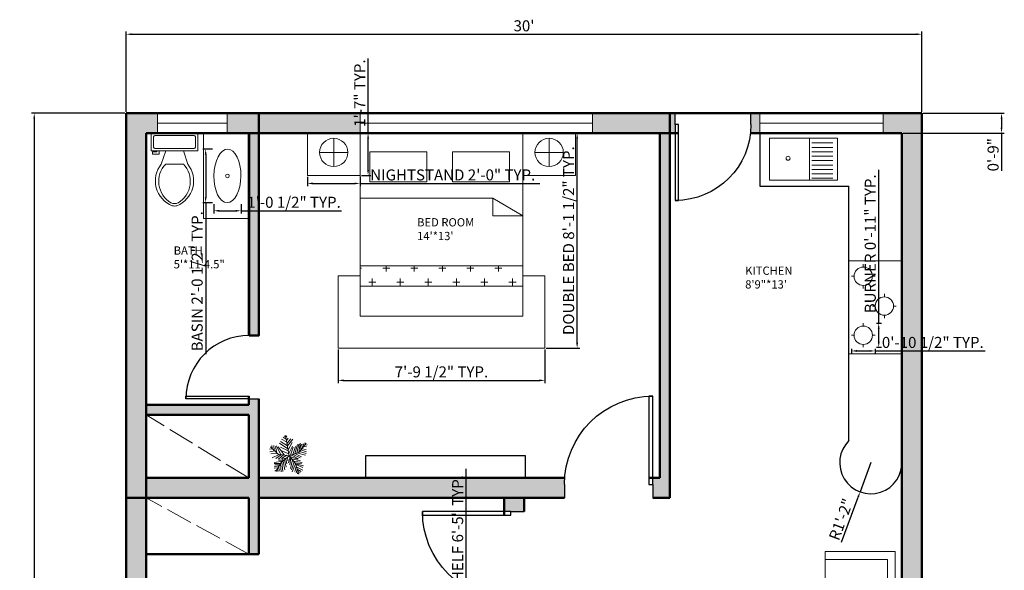
# Model space of a CAD drawing. Units: inches. Extents: x 1864 to 2313, y 963 to 1675.
# Tile 2 of 2: x 1868 to 2313, y 1425 to 1675. Entities that reach past the tile are written whole.
import ezdxf

# ---------------------------------------------------------------- set-up
doc = ezdxf.new("R2010")
doc.units = ezdxf.units.IN
doc.linetypes.add('ACAD_ISO02W100', pattern=[15, 12, -3])
for name, color, linetype, lineweight in [('A-ANNO-DIMS', 210, 'Continuous', 18), ('A-AREA-IDEN', 210, 'Continuous', 18), ('A-EQPM', 230, 'Continuous', 18), ('A-FLOR-CASE', 230, 'Continuous', 25), ('A-FLOR-CASE-OVHD', 142, 'ACAD_ISO02W100', 18), ('A-FLOR-FIXT', 40, 'Continuous', 18), ('A-FURN-PATT', 40, 'Continuous', 13), ('A-WALL-PATT', 142, 'Continuous', 13), ('door', 50, 'Continuous', 25), ('fur', 40, 'Continuous', 18), ('tree', 90, 'Continuous', 18), ('wall', 7, 'Continuous', 50), ('wind', 201, 'Continuous', 20)]:
    doc.layers.add(name, color=color, linetype=linetype, lineweight=lineweight)
doc.styles.get("Standard").update_dxf_attribs({"font": 'arial.ttf'})
doc.dimstyles.new('ISO-25', dxfattribs={"dimtxt": 5, "dimasz": 2.5, "dimexe": 1.25, "dimexo": 0.625, "dimtad": 1, "dimdec": 0, "dimlunit": 4, "dimtxsty": 'Standard', "dimcen": 2.5, "dimadec": 0, "dimazin": 0, "dimtfac": 1, "dimtdec": 0, "dimtmove": 0, "dimatfit": 3, "dimfxl": 1, "dimarcsym": 0})

# ---------------------------------------------------------------- blocks, each defined once
blk = doc.blocks.new('*U2')
for p, q in [((0, 0), (0, -6)), ((40, 0), (40, -6))]:
    blk.add_line(p, q)
blk.add_lwpolyline([(0, 0), (0, 40), (1.75, 40), (1.75, 0)], close=True)
blk.add_arc((0, 0), 40, 0, 90)
blk = doc.blocks.new('*U4')
for p, q in [((9.5, -6), (9.5, -2)), ((-10, -8.5), (-8, -8.5)), ((-10, -9.5), (-10, -8.5)), ((-8, -8.5), (-8, -8)), ((-7, -8), (-7, -9.5)), ((-4, -8), (-6, -14)), ((4, -8), (6, -14)), ((-7, -9.5), (-10, -9.5)), ((4, -14), (-4, -14))]:
    blk.add_line(p, q)
blk.add_lwpolyline([(10.5, -8), (10.5, 0), (-10.5, 0), (-10.5, -8)], close=True)
for points in [[(-9.5, -2), (-9.5, -6)], [(8.5, -1), (-8.5, -1)], [(-8.5, -7), (8.5, -7)]]:
    blk.add_lwpolyline(points)
for centre, radius, start, end in [((-8.62, -1.88), 0.884, 81.8699, 188.1301), ((8.62, -1.88), 0.884, 351.8699, 98.1301), ((-8.62, -6.12), 0.884, 171.8699, 278.1301), ((8.62, -6.12), 0.884, 261.8699, 8.1301), ((3.52, -21.58), 12.17, 141.4691, 247.9714), ((4.2, -21.82), 11.33, 136.3677, 238.9468), ((-3.52, -21.58), 12.17, 292.0284, 38.5307), ((-4.2, -21.82), 11.33, 301.053, 43.6321), ((0, -27.88), 4, 245.7318, 294.2682), ((0, -29), 4, 254.8605, 285.1395)]:
    blk.add_arc(centre, radius, start, end)
blk = doc.blocks.new('*U8')
for p, q in [((-10.186, 53.64), (-13.084, 55.962)), ((0, 0), (-10.5, 57)), ((-9.099, 51.782), (-6.563, 55.962)), ((-48.585, 21.131), (-49.309, 29.026)), ((-43.513, 28.561), (-42.427, 15.558)), ((-35.544, 28.097), (-24.314, 3.947)), ((-3.665, 19.273), (-27.574, 35.527)), ((-5.114, 28.097), (-24.676, 40.636)), ((-7.288, 39.707), (-21.778, 46.673)), ((-8.737, 47.138), (-17.069, 52.711)), ((-7.65, 43.423), (-2.578, 49.46)), ((-5.839, 35.992), (4.667, 48.067)), ((-5.114, 27.632), (10.463, 46.673)), ((-2.941, 16.486), (8.652, 37.85)), ((16.259, 5.805), (23.142, 31.348)), ((22.055, 7.198), (27.489, 32.277)), ((27, 9), (48, 36)), ((27.127, 9.056), (31.112, 35.992)), ((31.836, 30.883), (32.561, 16.486)), ((35.096, 32.741), (37.27, 22.524)), ((38.719, 34.134), (41.979, 28.561)), ((43.791, 29.954), (51.036, 30.883)), ((44.153, 36.456), (45.239, 32.741)), ((-47.498, 19.737), (-55.83, 18.344)), ((-40.615, 13.7), (-55.105, 10.913)), ((-31.5, 4.5), (-52.5, 25.5)), ((-33.37, 6.269), (-52.207, 5.34)), ((-28.299, 3.483), (-47.86, -5.805)), ((-38.442, 26.239), (-34.819, 7.663)), ((-21.416, 3.018), (-38.079, -8.128)), ((0, 0), (-31.5, 4.5)), ((-14.533, 2.09), (-30.834, 25.31)), ((-15.982, 2.09), (-30.11, -9.521)), ((-24.314, 23.917), (-2.941, 13.7)), ((0, 0), (-22.5, -19.5)), ((-6.563, 1.161), (-21.416, -8.128)), ((-20.691, 13.7), (-1.129, 4.876)), ((-1.129, 6.734), (9.014, 26.704)), ((0, 0), (27, 9)), ((0, 0), (18, -22.5)), ((3.942, 1.625), (11.187, 24.381)), ((6.478, 1.625), (26.04, -8.592)), ((10.101, 3.483), (17.708, 26.239)), ((11.187, 3.483), (30.749, -5.805)), ((18.07, 5.805), (35.096, -3.483)), ((24.229, 7.663), (46.688, 1.625)), ((29.662, 12.307), (48.137, 6.269)), ((33.285, 16.486), (48.862, 10.913)), ((36.183, 19.737), (48.137, 17.88)), ((40.53, 25.775), (48.862, 24.846)), ((-17.431, -15.094), (-42.789, -18.809)), ((-24.314, -21.596), (-42.427, -22.06)), ((-26.849, -26.24), (-40.253, -25.775)), ((-22.5, -19.5), (-37.5, -45)), ((-15.257, -12.772), (-30.11, -12.772)), ((-25.038, -23.918), (-22.865, -45.281)), ((-20.691, -18.345), (-17.793, -44.352)), ((-6.563, -5.805), (-19.967, -9.985)), ((-17.069, -15.094), (-12.721, -40.172)), ((-13.446, -11.378), (-8.737, -32.741)), ((-9.461, -8.592), (-6.201, -23.453)), ((-4.752, -3.483), (-3.665, -14.629)), ((2.493, -3.019), (-1.491, -20.202)), ((1.769, -2.555), (24.229, -9.521)), ((5.029, -6.27), (2.131, -25.775)), ((9.014, -11.378), (3.58, -35.992)), ((14.085, -16.951), (6.478, -40.172)), ((7.565, -9.056), (32.198, -14.629)), ((18.07, -22.524), (8.289, -45.745)), ((12.274, -15.094), (36.907, -18.809)), ((16.259, -19.738), (36.183, -22.989)), ((18, -22.5), (27, -52.5)), ((18.433, -22.524), (40.53, -29.026)), ((19.157, -25.311), (38.719, -33.206)), ((-28.299, -29.026), (-42.789, -31.348)), ((-30.834, -34.135), (-42.427, -35.528)), ((-34.457, -39.708), (-40.978, -42.494)), ((-32.646, -36.921), (-31.921, -44.352)), ((-29.023, -30.884), (-27.936, -43.887)), ((20.244, -30.419), (15.897, -44.816)), ((22.78, -37.85), (19.519, -48.532)), ((21.331, -32.741), (39.081, -40.636)), ((22.78, -38.314), (34.372, -44.816)), ((24.591, -45.745), (23.142, -50.854)), ((24.591, -43.423), (30.749, -47.603)), ((26.764, -49.925), (28.213, -50.854))]:
    blk.add_line(p, q)
blk = doc.blocks.new('*D9')
at = {"layer": 'A-ANNO-DIMS', "color": 0, "lineweight": -2, "transparency": 16777216}
for p, q in [((1915.95, 1632.78), (1915.95, 1669.17)), ((1918.45, 1667.92), (2273.45, 1667.92)), ((2275.95, 1632.78), (2275.95, 1669.17))]:
    blk.add_line(p, q, dxfattribs=at)
at = {"layer": 'A-ANNO-DIMS', "color": 0, "lineweight": 100, "transparency": 16777216}
for points in [[(1918.45, 1668.34), (1918.45, 1667.51), (1915.95, 1667.92)], [(2273.45, 1668.34), (2273.45, 1667.51), (2275.95, 1667.92)]]:
    blk.add_solid(points, dxfattribs=at)
at = {"layer": 'Defpoints', "color": 0, "lineweight": 100, "transparency": 16777216}
for p in [(2275.95, 1667.92), (1915.95, 1632.16), (2275.95, 1632.16)]:
    blk.add_point(p, dxfattribs=at)
at = {"layer": 'A-ANNO-DIMS', "color": 0, "transparency": 16777216, "insert": (2095.95, 1671.1), "char_height": 5, "attachment_point": 5}
blk.add_mtext("30'", dxfattribs=at)
blk = doc.blocks.new('*D10')
at = {"layer": 'A-ANNO-DIMS', "color": 0, "lineweight": -2, "transparency": 16777216}
for p, q in [((1915.33, 1632.16), (1873.06, 1632.16)), ((1874.31, 1629.66), (1874.31, 965.66)), ((1915.33, 963.16), (1873.06, 963.16))]:
    blk.add_line(p, q, dxfattribs=at)
at = {"layer": 'A-ANNO-DIMS', "color": 0, "lineweight": 100, "transparency": 16777216}
for points in [[(1873.89, 1629.66), (1874.73, 1629.66), (1874.31, 1632.16)], [(1873.89, 965.66), (1874.73, 965.66), (1874.31, 963.16)]]:
    blk.add_solid(points, dxfattribs=at)
at = {"layer": 'Defpoints', "color": 0, "lineweight": 100, "transparency": 16777216}
for p in [(1915.95, 1632.16), (1874.31, 963.16), (1915.95, 963.16)]:
    blk.add_point(p, dxfattribs=at)
at = {"layer": 'A-ANNO-DIMS', "color": 0, "transparency": 16777216, "insert": (1871.13, 1297.66), "char_height": 5, "attachment_point": 5, "rotation": 90}
blk.add_mtext('55\'-9"', dxfattribs=at)
blk = doc.blocks.new('BED-DOUBLE')
for p, q in [((10, 67.81), (70, 67.81)), ((70, 67.81), (70, 59.9)), ((83.6, 59.9), (70, 67.81)), ((70, 59.9), (83.6, 59.9)), ((5, 32.66), (0, 32.66)), ((0, 32.66), (0, 0)), ((10, 32.66), (5, 32.66)), ((83.6, 32.66), (93.6, 32.66)), ((93.6, 32.66), (93.6, 0)), ((0, 0), (93.6, 0))]:
    blk.add_line(p, q)
for points in [[(10, 97.3), (83.6, 97.3), (83.6, 14.55), (10, 14.55)], [(14.44, 88.9), (40.24, 88.9), (40.24, 75.28), (14.44, 75.28)], [(51.82, 88.9), (77.62, 88.9), (77.62, 75.28), (51.82, 75.28)]]:
    blk.add_lwpolyline(points, close=True)
blk = doc.blocks.new('TABLE-BEDSIDE')
for p, q in [((11.93, 4.03), (11.93, 16.85)), ((5.53, 10.44), (18.34, 10.44))]:
    blk.add_line(p, q)
blk.add_lwpolyline([(0, 19.17), (23.88, 19.17), (23.88, 0), (0, 0)], close=True)
blk.add_circle((11.93, 10.44), 6.41)
blk = doc.blocks.new('LOUNGE-CHAIR')
for p, q in [((3.79, 31.54), (0, 31.54)), ((0, 31.54), (0, 0)), ((3.79, 3.47), (3.79, 31.54)), ((30.24, 31.54), (33.95, 31.54)), ((33.95, 31.54), (33.95, 0)), ((0, 0), (33.95, 0))]:
    blk.add_line(p, q)
blk.add_lwpolyline([(3.79, 31.54), (30.24, 31.54), (30.24, 3.47), (3.79, 3.47)])
blk = doc.blocks.new('BASIN-OVAL')
blk.add_circle((12.11, 6.1), 0.811)
blk.add_ellipse((12.11, 6.1), major_axis=(12.1, -0.16), ratio=0.504372)
blk = doc.blocks.new('COOKTOP-BURNER')
for p, q in [((5.36, 10.94), (5.36, 9.63)), ((0, 5.47), (1.19, 5.47)), ((9.52, 5.47), (10.71, 5.47)), ((5.36, 1.31), (5.36, 0))]:
    blk.add_line(p, q)
blk.add_circle((5.36, 5.47), 4.16)
blk = doc.blocks.new('*D18')
at = {"layer": 'A-ANNO-DIMS', "color": 0, "lineweight": -2, "transparency": 16777216}
for p, q in [((1997.91, 1603.36), (1997.91, 1599.15)), ((2000.41, 1600.4), (2019.29, 1600.4)), ((2021.79, 1603.36), (2021.79, 1599.15)), ((2021.79, 1600.4), (2103.12, 1600.4))]:
    blk.add_line(p, q, dxfattribs=at)
at = {"layer": 'A-ANNO-DIMS', "color": 0, "lineweight": 100, "transparency": 16777216}
for points in [[(2000.41, 1600.82), (2000.41, 1599.99), (1997.91, 1600.4)], [(2019.29, 1600.82), (2019.29, 1599.99), (2021.79, 1600.4)]]:
    blk.add_solid(points, dxfattribs=at)
at = {"layer": 'Defpoints', "color": 0, "lineweight": 100, "transparency": 16777216}
for p in [(1997.91, 1603.99), (2021.79, 1603.99), (2021.79, 1600.4)]:
    blk.add_point(p, dxfattribs=at)
at = {"layer": 'A-ANNO-DIMS', "color": 0, "transparency": 16777216, "insert": (2063.71, 1603.61), "char_height": 5, "attachment_point": 5}
blk.add_mtext('NIGHTSTAND 2\'-0" TYP.', dxfattribs=at)
blk = doc.blocks.new('*D19')
at = {"layer": 'A-ANNO-DIMS', "color": 0, "lineweight": -2, "transparency": 16777216}
for p, q in [((2025.38, 1623.16), (2025.38, 1656.91)), ((2022.42, 1623.16), (2026.63, 1623.16)), ((2025.38, 1606.49), (2025.38, 1620.66)), ((2022.42, 1603.99), (2026.63, 1603.99))]:
    blk.add_line(p, q, dxfattribs=at)
at = {"layer": 'A-ANNO-DIMS', "color": 0, "lineweight": 100, "transparency": 16777216}
for points in [[(2024.96, 1620.66), (2025.79, 1620.66), (2025.38, 1623.16)], [(2024.96, 1606.49), (2025.79, 1606.49), (2025.38, 1603.99)]]:
    blk.add_solid(points, dxfattribs=at)
at = {"layer": 'Defpoints', "color": 0, "lineweight": 100, "transparency": 16777216}
for p in [(2021.79, 1623.16), (2025.38, 1623.16), (2021.79, 1603.99)]:
    blk.add_point(p, dxfattribs=at)
at = {"layer": 'A-ANNO-DIMS', "color": 0, "transparency": 16777216, "insert": (2022.24, 1641.28), "char_height": 5, "attachment_point": 5, "rotation": 90}
blk.add_mtext('1\'-7" TYP.', dxfattribs=at)
blk = doc.blocks.new('*D20')
at = {"layer": 'A-ANNO-DIMS', "color": 0, "lineweight": -2, "transparency": 16777216}
for p, q in [((2256.46, 1537.18), (2256.46, 1606.51)), ((2255.45, 1537.18), (2257.71, 1537.18)), ((2256.46, 1528.74), (2256.46, 1534.68)), ((2255.45, 1526.24), (2257.71, 1526.24))]:
    blk.add_line(p, q, dxfattribs=at)
at = {"layer": 'A-ANNO-DIMS', "color": 0, "lineweight": 100, "transparency": 16777216}
for points in [[(2256.05, 1534.68), (2256.88, 1534.68), (2256.46, 1537.18)], [(2256.05, 1528.74), (2256.88, 1528.74), (2256.46, 1526.24)]]:
    blk.add_solid(points, dxfattribs=at)
at = {"layer": 'Defpoints', "color": 0, "lineweight": 100, "transparency": 16777216}
for p in [(2254.82, 1537.18), (2256.46, 1537.18), (2254.82, 1526.24)]:
    blk.add_point(p, dxfattribs=at)
at = {"layer": 'A-ANNO-DIMS', "color": 0, "transparency": 16777216, "insert": (2253.29, 1573.09), "char_height": 5, "attachment_point": 5, "rotation": 90}
blk.add_mtext('BURNER 0\'-11" TYP.', dxfattribs=at)
blk = doc.blocks.new('*D21')
at = {"layer": 'A-ANNO-DIMS', "color": 0, "lineweight": -2, "transparency": 16777216}
for p, q in [((2244.11, 1525.62), (2244.11, 1523.35)), ((2246.61, 1524.6), (2252.32, 1524.6)), ((2254.82, 1525.62), (2254.82, 1523.35)), ((2254.82, 1524.6), (2304.59, 1524.6))]:
    blk.add_line(p, q, dxfattribs=at)
at = {"layer": 'A-ANNO-DIMS', "color": 0, "lineweight": 100, "transparency": 16777216}
for points in [[(2246.61, 1525.02), (2246.61, 1524.18), (2244.11, 1524.6)], [(2252.32, 1525.02), (2252.32, 1524.18), (2254.82, 1524.6)]]:
    blk.add_solid(points, dxfattribs=at)
at = {"layer": 'Defpoints', "color": 0, "lineweight": 100, "transparency": 16777216}
for p in [(2244.11, 1526.24), (2254.82, 1526.24), (2254.82, 1524.6)]:
    blk.add_point(p, dxfattribs=at)
at = {"layer": 'A-ANNO-DIMS', "color": 0, "transparency": 16777216, "insert": (2280.95, 1527.81), "char_height": 5, "attachment_point": 5}
blk.add_mtext('0\'-10 1/2" TYP.', dxfattribs=at)
blk = doc.blocks.new('*D22')
at = {"layer": 'A-ANNO-DIMS', "color": 0, "lineweight": -2, "transparency": 16777216}
for p, q in [((2106.01, 1623.16), (2121.23, 1623.16)), ((2119.98, 1528.36), (2119.98, 1620.66)), ((2106.01, 1525.86), (2121.23, 1525.86))]:
    blk.add_line(p, q, dxfattribs=at)
at = {"layer": 'A-ANNO-DIMS', "color": 0, "lineweight": 100, "transparency": 16777216}
for points in [[(2119.56, 1620.66), (2120.4, 1620.66), (2119.98, 1623.16)], [(2119.56, 1528.36), (2120.4, 1528.36), (2119.98, 1525.86)]]:
    blk.add_solid(points, dxfattribs=at)
at = {"layer": 'Defpoints', "color": 0, "lineweight": 100, "transparency": 16777216}
for p in [(2105.39, 1623.16), (2119.98, 1623.16), (2105.39, 1525.86)]:
    blk.add_point(p, dxfattribs=at)
at = {"layer": 'A-ANNO-DIMS', "color": 0, "transparency": 16777216, "insert": (2116.77, 1574.51), "char_height": 5, "attachment_point": 5, "rotation": 90}
blk.add_mtext('DOUBLE BED 8\'-1 1/2" TYP.', dxfattribs=at)
blk = doc.blocks.new('*D23')
at = {"layer": 'A-ANNO-DIMS', "color": 0, "lineweight": -2, "transparency": 16777216}
for p, q in [((2011.79, 1525.24), (2011.79, 1510.02)), ((2105.39, 1525.24), (2105.39, 1510.02)), ((2014.29, 1511.27), (2102.89, 1511.27))]:
    blk.add_line(p, q, dxfattribs=at)
at = {"layer": 'A-ANNO-DIMS', "color": 0, "lineweight": 100, "transparency": 16777216}
for points in [[(2014.29, 1511.69), (2014.29, 1510.85), (2011.79, 1511.27)], [(2102.89, 1511.69), (2102.89, 1510.85), (2105.39, 1511.27)]]:
    blk.add_solid(points, dxfattribs=at)
at = {"layer": 'Defpoints', "color": 0, "lineweight": 100, "transparency": 16777216}
for p in [(2011.79, 1525.86), (2105.39, 1525.86), (2105.39, 1511.27)]:
    blk.add_point(p, dxfattribs=at)
at = {"layer": 'A-ANNO-DIMS', "color": 0, "transparency": 16777216, "insert": (2058.59, 1514.48), "char_height": 5, "attachment_point": 5}
blk.add_mtext('7\'-9 1/2" TYP.', dxfattribs=at)
blk = doc.blocks.new('*D28')
at = {"layer": 'A-ANNO-DIMS', "color": 0, "lineweight": -2, "transparency": 16777216}
for p, q in [((1954.91, 1615.97), (1950.64, 1615.97)), ((1951.89, 1613.47), (1951.89, 1594.17)), ((1954.91, 1591.67), (1950.64, 1591.67)), ((1951.89, 1591.67), (1951.89, 1523.11))]:
    blk.add_line(p, q, dxfattribs=at)
at = {"layer": 'A-ANNO-DIMS', "color": 0, "lineweight": 100, "transparency": 16777216}
for points in [[(1951.48, 1613.47), (1952.31, 1613.47), (1951.89, 1615.97)], [(1951.48, 1594.17), (1952.31, 1594.17), (1951.89, 1591.67)]]:
    blk.add_solid(points, dxfattribs=at)
at = {"layer": 'Defpoints', "color": 0, "lineweight": 100, "transparency": 16777216}
for p in [(1955.54, 1615.97), (1951.89, 1591.67), (1955.54, 1591.67)]:
    blk.add_point(p, dxfattribs=at)
at = {"layer": 'A-ANNO-DIMS', "color": 0, "transparency": 16777216, "insert": (1948.68, 1556.14), "char_height": 5, "attachment_point": 5, "rotation": 90}
blk.add_mtext('BASIN 2\'-0 1/2" TYP.', dxfattribs=at)
blk = doc.blocks.new('*D29')
at = {"layer": 'A-ANNO-DIMS', "color": 0, "lineweight": -2, "transparency": 16777216}
for p, q in [((1955.54, 1591.05), (1955.54, 1586.78)), ((1967.93, 1591.05), (1967.93, 1586.78)), ((1958.04, 1588.03), (1965.43, 1588.03)), ((1967.93, 1588.03), (2013.33, 1588.03))]:
    blk.add_line(p, q, dxfattribs=at)
at = {"layer": 'A-ANNO-DIMS', "color": 0, "lineweight": 100, "transparency": 16777216}
for points in [[(1958.04, 1588.44), (1958.04, 1587.61), (1955.54, 1588.03)], [(1965.43, 1588.44), (1965.43, 1587.61), (1967.93, 1588.03)]]:
    blk.add_solid(points, dxfattribs=at)
at = {"layer": 'Defpoints', "color": 0, "lineweight": 100, "transparency": 16777216}
for p in [(1955.54, 1591.67), (1967.93, 1591.67), (1967.93, 1588.03)]:
    blk.add_point(p, dxfattribs=at)
at = {"layer": 'A-ANNO-DIMS', "color": 0, "transparency": 16777216, "insert": (1991.88, 1591.24), "char_height": 5, "attachment_point": 5}
blk.add_mtext('1\'-0 1/2" TYP.', dxfattribs=at)
blk = doc.blocks.new('*D30')
at = {"layer": 'A-ANNO-DIMS', "color": 0, "lineweight": -2, "transparency": 16777216}
for p, q in [((2069.78, 1391.45), (2069.78, 1471.3)), ((2080.73, 1391.45), (2068.53, 1391.45)), ((2069.78, 1316.78), (2069.78, 1388.95)), ((2080.73, 1314.28), (2068.53, 1314.28))]:
    blk.add_line(p, q, dxfattribs=at)
at = {"layer": 'A-ANNO-DIMS', "color": 0, "lineweight": 100, "transparency": 16777216}
for points in [[(2069.36, 1388.95), (2070.19, 1388.95), (2069.78, 1391.45)], [(2069.36, 1316.78), (2070.19, 1316.78), (2069.78, 1314.28)]]:
    blk.add_solid(points, dxfattribs=at)
at = {"layer": 'Defpoints', "color": 0, "lineweight": 100, "transparency": 16777216}
for p in [(2069.78, 1391.45), (2081.35, 1391.45), (2081.35, 1314.28)]:
    blk.add_point(p, dxfattribs=at)
at = {"layer": 'A-ANNO-DIMS', "color": 0, "transparency": 16777216, "insert": (2066.57, 1432.63), "char_height": 5, "attachment_point": 5, "rotation": 90}
blk.add_mtext('WALL SHELF 6\'-5" TYP.', dxfattribs=at)
blk = doc.blocks.new('*D32')
at = {"layer": 'A-ANNO-DIMS', "color": 0, "lineweight": -2, "transparency": 16777216}
for p, q in [((2276.58, 1632.16), (2313.3, 1632.16)), ((2312.05, 1629.66), (2312.05, 1625.66)), ((2267.58, 1623.16), (2313.3, 1623.16)), ((2312.05, 1623.16), (2312.05, 1606.11))]:
    blk.add_line(p, q, dxfattribs=at)
at = {"layer": 'A-ANNO-DIMS', "color": 0, "lineweight": 100, "transparency": 16777216}
for points in [[(2311.64, 1629.66), (2312.47, 1629.66), (2312.05, 1632.16)], [(2311.64, 1625.66), (2312.47, 1625.66), (2312.05, 1623.16)]]:
    blk.add_solid(points, dxfattribs=at)
at = {"layer": 'Defpoints', "color": 0, "lineweight": 100, "transparency": 16777216}
for p in [(2275.95, 1632.16), (2266.95, 1623.16), (2312.05, 1623.16)]:
    blk.add_point(p, dxfattribs=at)
at = {"layer": 'A-ANNO-DIMS', "color": 0, "transparency": 16777216, "insert": (2308.88, 1613.39), "char_height": 5, "attachment_point": 5, "rotation": 90}
blk.add_mtext('0\'-9"', dxfattribs=at)
blk = doc.blocks.new('*D33')
at = {"layer": 'A-ANNO-DIMS', "color": 0, "lineweight": -2, "transparency": 16777216}
for p, q in [((2252.91, 1474.05), (2248.04, 1460.83)), ((2239.64, 1438), (2247.18, 1458.48))]:
    blk.add_line(p, q, dxfattribs=at)
at = {"layer": 'A-ANNO-DIMS', "color": 0, "lineweight": 100, "transparency": 16777216}
blk.add_solid([(2246.79, 1458.63), (2247.57, 1458.34), (2248.04, 1460.83)], dxfattribs=at)
at = {"layer": 'Defpoints', "color": 0, "lineweight": 100, "transparency": 16777216}
for p in [(2252.91, 1474.05), (2248.04, 1460.83)]:
    blk.add_point(p, dxfattribs=at)
at = {"layer": 'A-ANNO-DIMS', "color": 0, "transparency": 16777216, "insert": (2240.03, 1448.15), "char_height": 5, "attachment_point": 5, "rotation": 69.7872}
blk.add_mtext('R1\'-2"', dxfattribs=at)

msp = doc.modelspace()

# ---------------------------------------------------------------- hatches: boundary and pattern name
at = {"layer": 'A-FURN-PATT'}
h = msp.add_hatch(dxfattribs=at)
h.set_pattern_fill('CROSS', color=256)
h.paths.add_polyline_path([(2095.39, 1563.09), (2021.79, 1563.09), (2021.79, 1553.95), (2095.39, 1553.95)])
at = {"layer": 'A-WALL-PATT'}
h = msp.add_hatch(color=256, dxfattribs=at)
h.dxf.hatch_style = 1
h.paths.add_polyline_path([(1975.95, 1632.16), (1961.64, 1632.16), (1961.64, 1623.16), (1971.45, 1623.16), (1975.95, 1623.16)])
h.paths.add_polyline_path([(2021.79, 1632.16), (1989.45, 1632.16), (1975.95, 1632.16), (1975.95, 1623.16), (1984.95, 1623.16), (1989.45, 1623.16), (2021.79, 1623.16)])
h.paths.add_polyline_path([(2161.95, 1632.16), (2126.93, 1632.16), (2126.93, 1623.16), (2157.45, 1623.16), (2161.95, 1623.16)])
h.paths.add_polyline_path([(2275.95, 1632.16), (2258.45, 1632.16), (2258.45, 1623.16), (2266.95, 1623.16), (2266.95, 1475.18, -0.040334), (2266.95, 1472.91), (2266.95, 1467.16), (2266.95, 1458.16), (2266.95, 1278.16), (2266.95, 1269.16), (2275.95, 1269.16), (2275.95, 1458.16)])
h.paths.add_polyline_path([(2161.95, 1623.16), (2157.45, 1623.16), (2157.45, 1467.16), (2154.26, 1467.16), (2154.26, 1464.16), (2154.26, 1458.16), (2161.95, 1458.16)])
h.paths.add_polyline_path([(2202.62, 1632.16), (2198.67, 1632.16), (2198.67, 1627.01, -0.028105), (2198.46, 1623.16), (2202.62, 1623.16)])
h.paths.add_polyline_path([(2164.34, 1627.01), (2164.34, 1632.16), (2161.95, 1632.16), (2161.95, 1623.16), (2164.34, 1623.16)])
h.paths.add_polyline_path([(1930.16, 1632.16), (1929.45, 1632.16), (1915.95, 1632.16), (1915.95, 1458.16), (1924.95, 1458.16), (1924.95, 1623.16), (1930.16, 1623.16)])
h.paths.add_polyline_path([(1924.95, 1441.66), (1924.95, 1458.16), (1915.95, 1458.16), (1915.95, 1285.66), (1924.95, 1285.66)])
h.paths.add_polyline_path([(2044.94, 1221.16), (2037.45, 1221.16), (1924.95, 1221.16), (1924.95, 1216.66), (2044.94, 1216.66)])
h.paths.add_polyline_path([(2037.45, 1234.15), (2032.95, 1234.15), (2032.95, 1221.16), (2037.45, 1221.16)])
h.paths.add_polyline_path([(2086.95, 1221.16), (2076.95, 1221.16), (2076.95, 1216.66), (2086.95, 1216.66)])
h.paths.add_polyline_path([(2107.14, 1185.16), (2095.95, 1185.16), (2095.95, 1189.94), (2092.08, 1189.94, -0.049915), (2086.95, 1190.46), (2086.95, 1176.16), (2107.14, 1176.16), (2107.14, 1178.61)])
h.paths.add_polyline_path([(2095.95, 1176.16), (2086.95, 1176.16), (2086.95, 1056.16), (2086.95, 1039.66), (2095.95, 1039.66), (2095.95, 1056.16)])
h.paths.add_polyline_path([(2086.95, 1048.66), (2057.44, 1048.66), (2057.44, 1039.66), (2086.95, 1039.66)])
h.paths.add_polyline_path([(1959.08, 1048.66), (1915.95, 1048.66), (1915.95, 1039.66), (1920.45, 1039.66), (1959.08, 1039.66)])
h.paths.add_polyline_path([(1924.95, 1216.66), (1924.95, 1221.16), (1915.95, 1221.16), (1915.95, 1048.66), (1924.95, 1048.66)])
h.paths.add_polyline_path([(1924.95, 1281.16), (1924.95, 1285.66), (1915.95, 1285.66), (1915.95, 1221.16), (1924.95, 1221.16)])
h.paths.add_polyline_path([(2037.45, 1285.66), (2028.44, 1285.66), (2028.44, 1281.58), (2028.44, 1281.16), (2032.95, 1281.16), (2032.95, 1272.41), (2037.45, 1272.41)])
h.paths.add_polyline_path([(2045.26, 1285.66), (2037.45, 1285.66), (2037.45, 1281.16), (2045.26, 1281.16)])
h.paths.add_polyline_path([(2086.95, 1285.66), (2080.03, 1285.66), (2080.03, 1281.16), (2086.95, 1281.16)])
h.paths.add_polyline_path([(2095.95, 1269.16), (2086.95, 1269.16), (2086.95, 1215.79), (2092.08, 1215.79), (2095.95, 1215.79)])
h = msp.add_hatch(color=256, dxfattribs=at)
h.dxf.hatch_style = 1
h.paths.add_polyline_path([(1975.95, 1623.16), (1971.64, 1623.16), (1971.64, 1531.6), (1975.95, 1531.6)])
h = msp.add_hatch(color=256, dxfattribs=at)
h.dxf.hatch_style = 1
h.paths.add_polyline_path([(1975.95, 1502.87), (1971.45, 1502.87), (1971.45, 1500.16), (1924.95, 1500.16), (1924.95, 1495.66), (1971.45, 1495.66), (1971.45, 1467.16), (1924.95, 1467.16), (1924.95, 1458.16), (1971.45, 1458.16), (1971.45, 1432.56), (1975.95, 1432.56), (1975.95, 1467.16)])
h.paths.add_polyline_path([(2114.37, 1467.16), (1975.95, 1467.16), (1975.95, 1458.16), (2114.26, 1458.16), (2114.26, 1464.16, -0.01877)])
h.paths.add_polyline_path([(2095.95, 1458.16), (2086.95, 1458.16), (2086.95, 1451.99), (2089.95, 1451.99), (2095.95, 1451.99)])

# ---------------------------------------------------------------- linework, layer by layer
at = {"layer": 'A-EQPM'}
msp.add_lwpolyline([(2266.95, 1565.31), (2242.95, 1565.31), (2242.95, 1523.35), (2266.95, 1523.35)], close=True, dxfattribs=at)
at = {"layer": 'A-FLOR-CASE'}
for p, q in [((2202.62, 1623.16), (2202.62, 1599.16)), ((2202.62, 1599.16), (2242.95, 1599.16)), ((2242.95, 1484.02), (2242.95, 1599.16))]:
    msp.add_line(p, q, dxfattribs=at)
msp.add_lwpolyline([(2024.23, 1467.16), (2096.59, 1467.16), (2096.59, 1477.17), (2024.23, 1477.17)], close=True, dxfattribs=at)
msp.add_arc((2252.91, 1474.05), 14.09, 134.9578, 4.6195, dxfattribs=at)
at = {"layer": 'A-FLOR-CASE-OVHD'}
for p, q in [((1971.45, 1467.16), (1924.95, 1495.66)), ((1971.45, 1432.56), (1924.95, 1458.16))]:
    msp.add_line(p, q, dxfattribs=at)
at = {"layer": 'A-FLOR-FIXT'}
for p, q in [((2225.19, 1601.88), (2225.19, 1620.84)), ((2226.15, 1618.72), (2235.74, 1618.72)), ((2226.15, 1616.72), (2235.74, 1616.72)), ((2226.15, 1614.72), (2235.74, 1614.72)), ((2226.15, 1612.72), (2235.74, 1612.72)), ((2226.15, 1610.72), (2235.74, 1610.72)), ((2226.15, 1608.72), (2235.74, 1608.72)), ((2226.15, 1606.72), (2235.74, 1606.72)), ((2226.15, 1604.72), (2235.74, 1604.72)), ((2226.15, 1602.72), (2235.74, 1602.72))]:
    msp.add_line(p, q, dxfattribs=at)
for points in [[(1971.45, 1623.16), (1971.45, 1584.47), (1950.84, 1584.47), (1950.84, 1623.16)], [(2207.04, 1620.84), (2237.78, 1620.84), (2237.78, 1601.88), (2207.04, 1601.88)]]:
    msp.add_lwpolyline(points, close=True, dxfattribs=at)
msp.add_circle((2215.43, 1611.82), 0.917, dxfattribs=at)
at = {"layer": 'fur'}
msp.add_lwpolyline([(2021.79, 1553.95), (2095.39, 1553.95), (2095.39, 1563.09), (2021.79, 1563.09)], close=True, dxfattribs=at)
at = {"layer": 'wall'}
for p, q in [((1915.95, 1495.66), (1915.95, 1632.16)), ((1915.95, 1285.66), (1915.95, 1632.16)), ((1915.95, 1632.16), (1929.45, 1632.16)), ((1929.45, 1632.16), (1989.45, 1632.16)), ((1975.95, 1632.16), (1975.95, 1531.6)), ((1989.45, 1632.16), (2161.95, 1632.16)), ((2161.95, 1632.16), (2161.95, 1458.16)), ((2161.95, 1632.16), (2275.95, 1632.16)), ((2275.95, 1632.16), (2275.95, 1458.16)), ((1924.95, 1623.16), (1984.95, 1623.16)), ((1924.95, 1500.16), (1924.95, 1623.16)), ((1924.95, 1281.16), (1924.95, 1623.16)), ((1971.45, 1623.16), (1971.45, 1531.6)), ((1975.95, 1623.16), (1975.95, 1531.6)), ((1984.95, 1623.16), (1989.45, 1623.16)), ((1989.45, 1623.16), (2157.45, 1623.16)), ((2157.45, 1623.16), (2157.45, 1467.16)), ((2157.45, 1623.16), (2161.95, 1623.16)), ((2161.95, 1623.16), (2165.84, 1623.16)), ((2198.46, 1623.16), (2266.95, 1623.16)), ((2266.95, 1623.16), (2266.95, 1467.16)), ((1971.45, 1504.13), (1971.45, 1500.16)), ((1975.95, 1502.87), (1975.95, 1467.16)), ((1975.95, 1502.87), (1975.95, 1495.66)), ((1971.45, 1500.16), (1924.95, 1500.16)), ((1915.95, 1495.66), (1915.95, 1458.16)), ((1971.45, 1495.66), (1924.95, 1495.66)), ((1924.95, 1495.66), (1924.95, 1467.16)), ((1971.45, 1467.16), (1971.45, 1495.66)), ((1975.95, 1467.16), (1975.95, 1495.66)), ((1971.45, 1467.16), (1971.45, 1472.45)), ((1975.95, 1467.16), (1975.95, 1472.45)), ((1971.45, 1467.16), (1924.95, 1467.16)), ((1975.95, 1467.16), (1975.95, 1432.56)), ((2114.37, 1467.16), (1975.95, 1467.16)), ((2157.45, 1467.16), (2152.51, 1467.16)), ((2266.95, 1467.16), (2266.95, 1458.16)), ((1971.45, 1458.16), (1915.95, 1458.16)), ((1971.45, 1458.16), (1971.45, 1432.56)), ((2114.26, 1458.16), (1975.95, 1458.16)), ((2086.95, 1450.24), (2086.95, 1458.16)), ((2095.95, 1451.99), (2095.95, 1458.16)), ((2161.95, 1458.16), (2154.26, 1458.16)), ((2266.95, 1458.16), (2266.95, 1278.16)), ((2275.95, 1458.16), (2275.95, 1269.16)), ((1924.95, 1285.66), (1924.95, 1441.66)), ((1971.45, 1432.56), (1924.95, 1432.56)), ((1927.7, 1432.56), (1924.95, 1432.56)), ((1975.95, 1432.56), (1971.45, 1432.56))]:
    msp.add_line(p, q, dxfattribs=at)
msp.add_lwpolyline([(1971.64, 1623.16), (1975.95, 1623.16), (1975.95, 1531.6), (1971.64, 1531.6)], close=True, dxfattribs=at)
at = {"layer": 'wind'}
for p, q in [((1930.16, 1627.66), (1961.64, 1627.66)), ((2021.79, 1627.66), (2126.93, 1627.66)), ((2202.62, 1627.66), (2258.45, 1627.66))]:
    msp.add_line(p, q, dxfattribs=at)
for points in [[(1930.16, 1623.16), (1961.64, 1623.16), (1961.64, 1632.16), (1930.16, 1632.16)], [(2021.79, 1623.16), (2126.93, 1623.16), (2126.93, 1632.16), (2021.79, 1632.16)], [(2258.45, 1632.16), (2202.62, 1632.16), (2202.62, 1623.16), (2258.45, 1623.16)]]:
    msp.add_lwpolyline(points, close=True, dxfattribs=at)

# ---------------------------------------------------------------- block references
at = {"layer": 'A-EQPM'}
for p in [(2244.11, 1552.92), (2253.67, 1539.46), (2244.11, 1526.24)]:
    msp.add_blockref('COOKTOP-BURNER', p, dxfattribs=at)
at = {"layer": 'A-FLOR-FIXT'}
msp.add_blockref('*U4', (1937.79, 1623.16), dxfattribs=at)
at = {"layer": 'A-FLOR-FIXT', "rotation": 269.9999999999978}
msp.add_blockref('BASIN-OVAL', (1955.63, 1615.93), dxfattribs=at)
at = {"layer": 'door'}
for p, xscale, yscale, zscale, rotation in [((2164.34, 1627.01), -0.858268468651503, 0.858268468651503, 0.858268468651503, 180), ((1971.64, 1502.87), 0.718277175322918, 0.718277175322918, 0.718277175322918, 90)]:
    msp.add_blockref('*U2', p, dxfattribs=dict(at, xscale=xscale, yscale=yscale, zscale=zscale, rotation=rotation))
at = {"layer": 'door', "xscale": -1}
msp.add_blockref('*U2', (2154.26, 1464.16), dxfattribs=at)
at = {"layer": 'door', "xscale": -1, "rotation": 90}
msp.add_blockref('*U2', (2089.95, 1451.99), dxfattribs=at)
at = {"layer": 'fur'}
for name, p in [('TABLE-BEDSIDE', (1997.91, 1603.99)), ('BED-DOUBLE', (2011.79, 1525.86)), ('TABLE-BEDSIDE', (2095.39, 1603.99))]:
    msp.add_blockref(name, p, dxfattribs=at)
at = {"layer": 'fur', "rotation": 89.99999999999964}
msp.add_blockref('LOUNGE-CHAIR', (2263.85, 1399.95), dxfattribs=at)
at = {"layer": 'tree', "xscale": 0.1597188363102572, "yscale": 0.1597188363102572, "zscale": 0.1597188363102572}
msp.add_blockref('*U8', (1989.68, 1477.18), dxfattribs=at)

# ---------------------------------------------------------------- texts
at = {"layer": 'A-AREA-IDEN', "char_height": 3.726, "attachment_point": 1}
for s, insert in [("BED ROOM\\P14'*13'", (2047.57, 1584.69)), ('BATH\\P5\'*11\'4.5"', (1937.41, 1571.9)), ('KITCHEN\\P8\'9"*13\'', (2196.04, 1562.79))]:
    msp.add_mtext_dynamic_manual_height_columns(s, width=46.4423, gutter_width=18.63, heights=[0], dxfattribs=dict(at, insert=insert))

# ---------------------------------------------------------------- dimensions: what is measured, and where the dimension line sits
at = {"layer": 'A-ANNO-DIMS'}
dim = msp.add_linear_dim(base=(2275.95, 1667.92), p1=(1915.95, 1632.16), p2=(2275.95, 1632.16), dimstyle='ISO-25', override={"dimclrd": 0, "dimclre": 0, "dimclrt": 0}, dxfattribs=at)
dim.commit()
dim.dimension.update_dxf_attribs({"geometry": '*D9', "text_midpoint": (2095.95, 1671.1)})
for base, p1, p2, angle, text, picture, middle in [((2025.38, 1623.16), (2021.79, 1603.99), (2021.79, 1623.16), 90, '<> TYP.', '*D19', (2022.24, 1641.28)), ((2119.98, 1623.16), (2105.39, 1525.86), (2105.39, 1623.16), 90, 'DOUBLE BED <> TYP.', '*D22', (2116.77, 1574.51)), ((1951.89, 1591.67), (1955.54, 1615.97), (1955.54, 1591.67), 270, 'BASIN <> TYP.', '*D28', (1948.68, 1556.14)), ((2256.46, 1537.18), (2254.82, 1526.24), (2254.82, 1537.18), 90, 'BURNER <> TYP.', '*D20', (2253.29, 1573.09)), ((2069.78, 1391.45), (2081.35, 1314.28), (2081.35, 1391.45), 90, 'WALL SHELF <> TYP.', '*D30', (2066.57, 1432.63))]:
    dim = msp.add_linear_dim(base=base, p1=p1, p2=p2, angle=angle, text=text, dimstyle='ISO-25', override={"dimdec": 1, "dimlfac": 1, "dimrnd": 0, "dimzin": 1, "dimdsep": 46, "dimlunit": 4, "dimfrac": 2}, dxfattribs=at)
    dim.commit()
    dim.dimension.update_dxf_attribs({"geometry": picture, "text_midpoint": middle})
for base, p1, p2, override, picture, middle in [((1874.31, 963.16), (1915.95, 1632.16), (1915.95, 963.16), {"dimclrd": 0, "dimclre": 0, "dimclrt": 0}, '*D10', (1871.13, 1297.66)), ((2312.05, 1623.16), (2275.95, 1632.16), (2266.95, 1623.16), {"dimdec": 1, "dimlfac": 1, "dimrnd": 0, "dimzin": 1, "dimdsep": 46, "dimlunit": 4, "dimfrac": 2}, '*D32', (2308.88, 1613.39))]:
    dim = msp.add_linear_dim(base=base, p1=p1, p2=p2, angle=90, dimstyle='ISO-25', override=override, dxfattribs=at)
    dim.commit()
    dim.dimension.update_dxf_attribs({"geometry": picture, "text_midpoint": middle})
for base, p1, p2, text, picture, middle in [((2021.79, 1600.4), (1997.91, 1603.99), (2021.79, 1603.99), 'NIGHTSTAND <> TYP.', '*D18', (2063.71, 1603.61)), ((1967.93, 1588.03), (1955.54, 1591.67), (1967.93, 1591.67), '<> TYP.', '*D29', (1991.88, 1591.24)), ((2254.82, 1524.6), (2244.11, 1526.24), (2254.82, 1526.24), '<> TYP.', '*D21', (2280.95, 1527.81)), ((2105.39, 1511.27), (2011.79, 1525.86), (2105.39, 1525.86), '<> TYP.', '*D23', (2058.59, 1514.48))]:
    dim = msp.add_linear_dim(base=base, p1=p1, p2=p2, text=text, dimstyle='ISO-25', override={"dimdec": 1, "dimlfac": 1, "dimrnd": 0, "dimzin": 1, "dimdsep": 46, "dimlunit": 4, "dimfrac": 2}, dxfattribs=at)
    dim.commit()
    dim.dimension.update_dxf_attribs({"geometry": picture, "text_midpoint": middle})
dim = msp.add_radius_dim(center=(2252.91, 1474.05), mpoint=(2248.04, 1460.83), dimstyle='ISO-25', override={"dimdec": 1, "dimlfac": 1, "dimrnd": 0, "dimzin": 1, "dimdsep": 46, "dimlunit": 4, "dimfrac": 2}, dxfattribs=at)
dim.commit()
dim.dimension.update_dxf_attribs({"geometry": '*D33', "text_midpoint": (2240.03, 1448.15)})

doc.saveas('drawing.dxf')
